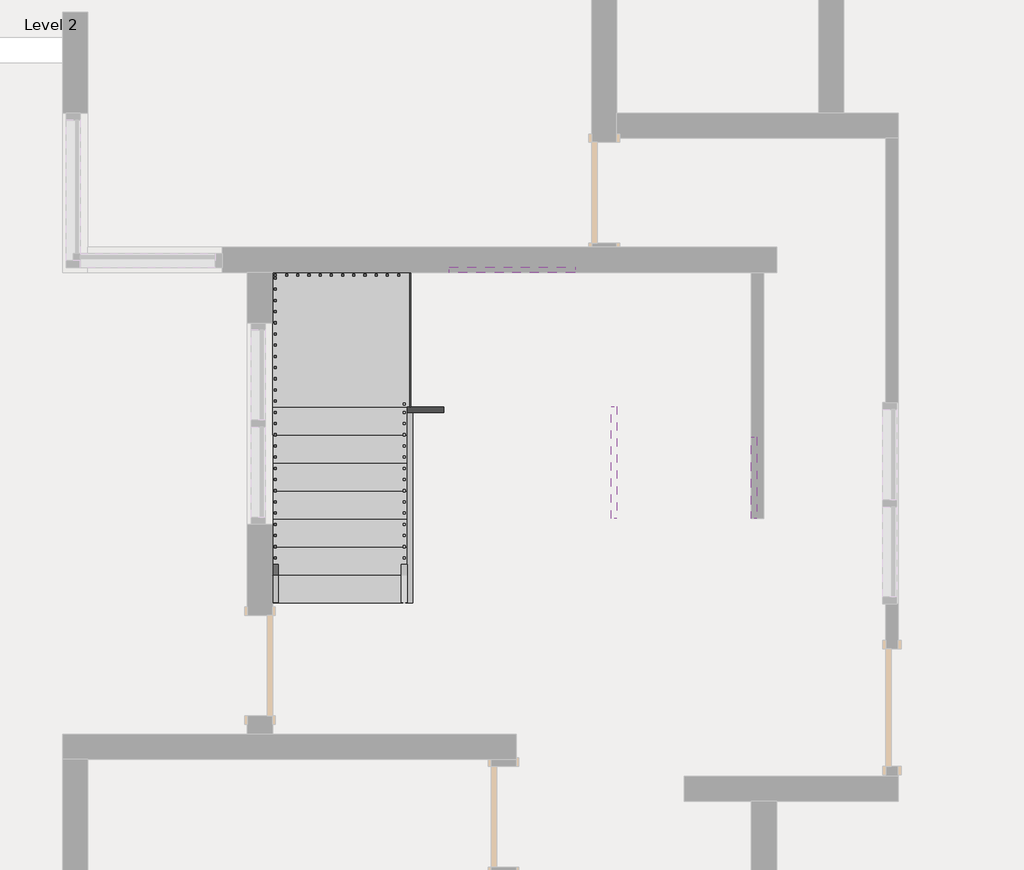
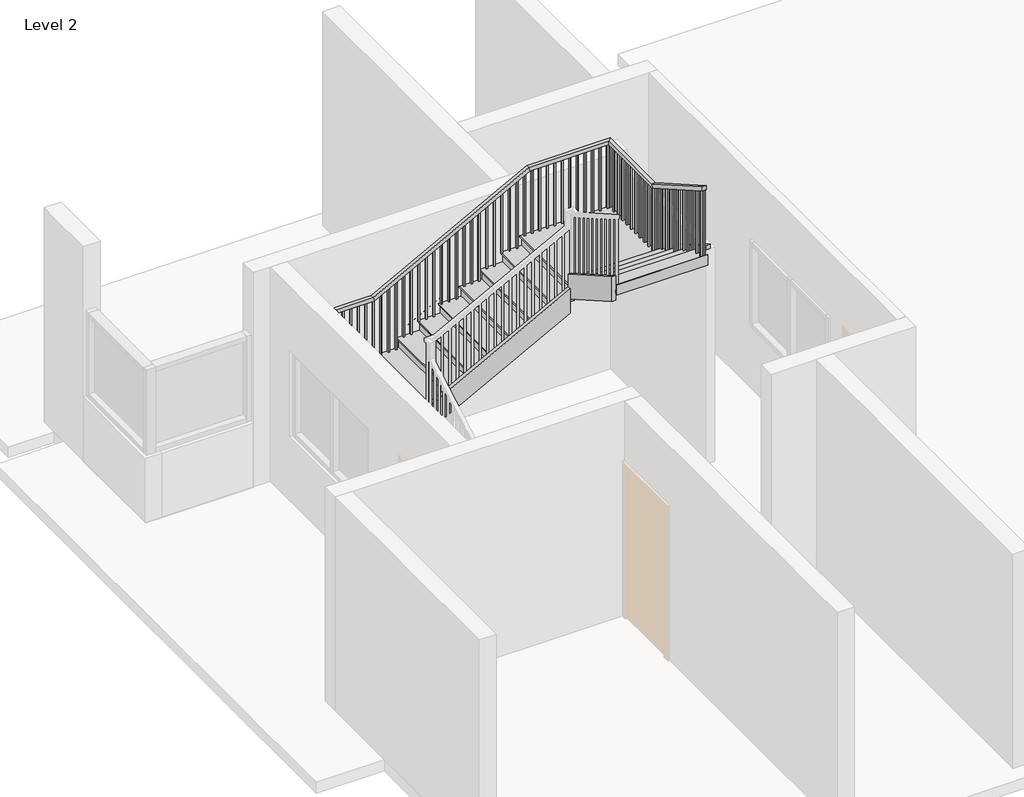
# One storey, part 5 of 5: 6 members, 1 railing, 1 stair flight.
"""IFC4 building model written with IfcOpenShell, lengths in millimetres."""

from ifc_helpers import new_model, si_unit, frame, origin, place, context, project, spatial, polyline, outline, extrude, faceted_brep, transform, mapped, element, save
from components import stair_flight_6f949d0f

model = new_model("IFC4")

# Units and contexts
model_context = context("Model", 3, world=origin())
ifc_project = project(units=[si_unit("LENGTHUNIT", "METRE", prefix="MILLI")], contexts=[model_context])

# Site, building, storey
site = spatial("IfcSite", under=ifc_project)
building = spatial("IfcBuilding", under=site)
storey = spatial("IfcBuildingStorey", under=building, Name="Level 2", Elevation=3048.0)

# Members
placement = place(None, origin())
element("IfcMember", 1, ObjectType="Stringer - 2\" Width", at=placement, inside=storey, context=model_context, shape_type="SweptSolid", body=[
    extrude(outline(polyline([(12459.3864709, 3048.0), (12459.3864709, 3256.974685), (13347.8057723, 3764.6428571), (13962.1498127, 3764.6428571), (12708.0248127, 3048.0), (12459.3864709, 3048.0)])), frame((-41052.5146233, 0.0, 0.0), z_axis=(1.0, 0.0, 0.0), x_axis=(0.0, 1.0, 0.0)), (0.0, 0.0, 1.0), 50.8),
])
element("IfcMember", 2, ObjectType="Stringer - 2\" Width", at=placement, inside=storey, context=model_context, shape_type="SweptSolid", body=[
    extrude(outline(polyline([(4618.6066619, -38752.8324895), (4882.574685, -38257.8924462), (4882.574685, -38905.5924462), (4618.6066619, -39400.5324895), (4618.6066619, -38752.8324895)])), frame((0.0, 15456.5864709, 0.0), z_axis=(0.0, 1.0, 0.0), x_axis=(0.0, 0.0, 1.0)), (0.0, 0.0, 1.0), 50.8),
])
element("IfcMember", 3, ObjectType="Stringer - 2\" Width", at=placement, inside=storey, context=model_context, shape_type="SweptSolid", body=[
    extrude(outline(polyline([(13349.3031292, 5735.6828571), (13221.3864709, 5808.7780904), (13221.3864709, 6159.8318278), (13963.6471696, 5735.6828571), (13349.3031292, 5735.6828571)])), frame((-36658.3146233, 0.0, 0.0), z_axis=(1.0, 0.0, 0.0), x_axis=(0.0, 1.0, 0.0)), (0.0, 0.0, 1.0), 50.8),
])
element("IfcMember", 4, ObjectType="Stringer - 2\" Width", at=placement, inside=storey, context=model_context, shape_type="SweptSolid", body=[
    extrude(outline(polyline([(12459.3864709, 3048.0), (12459.3864709, 3256.974685), (14186.5864709, 4243.9461135), (14186.5864709, 3892.8923761), (12708.0248127, 3048.0), (12459.3864709, 3048.0)])), frame((-39782.5146233, 0.0, 0.0), z_axis=(1.0, 0.0, 0.0), x_axis=(0.0, 1.0, 0.0)), (0.0, 0.0, 1.0), 50.8),
])
element("IfcMember", 5, ObjectType="Stringer - 2\" Width", at=placement, inside=storey, context=model_context, shape_type="SweptSolid", body=[
    extrude(outline(polyline([(4414.8828571, -39782.5146233), (4069.4428571, -39782.5146233), (5058.3495238, -37928.3146233), (5403.7895238, -37928.3146233), (4414.8828571, -39782.5146233)])), frame((0.0, 14186.5864709, 0.0), z_axis=(0.0, 1.0, 0.0), x_axis=(0.0, 0.0, 1.0)), (0.0, 0.0, 1.0), 50.8),
])
element("IfcMember", 6, ObjectType="Stringer - 2\" Width", at=placement, inside=storey, context=model_context, shape_type="SweptSolid", body=[
    extrude(outline(polyline([(14237.3864709, 5579.2603992), (14237.3864709, 5228.2066619), (13221.3864709, 5808.7780904), (13221.3864709, 6159.8318278), (14237.3864709, 5579.2603992)])), frame((-37928.3146233, 0.0, 0.0), z_axis=(1.0, 0.0, 0.0), x_axis=(0.0, 1.0, 0.0)), (0.0, 0.0, 1.0), 50.8),
])

# Railing
element("IfcRailing", 7, ObjectType="Handrail - Rectangular", at=placement, inside=storey, context=model_context, shape_type="SolidModel", body=[
    faceted_brep([(-41001.7146233, 12459.3864709, 4107.5428571), (-41001.7146233, 12459.3864709, 4049.0339009), (-40950.9146233, 12459.3864709, 4049.0339009), (-40950.9146233, 12459.3864709, 4107.5428571), (-41001.7146233, 14404.1798043, 5218.8533333), (-41001.7146233, 14417.6704777, 5168.0533333), (-40950.9146233, 14417.6704777, 5168.0533333), (-40950.9146233, 14404.1798043, 5218.8533333), (-41001.7146233, 15456.5864709, 5218.8533333), (-41001.7146233, 15456.5864709, 5168.0533333), (-40950.9146233, 15405.7864709, 5168.0533333), (-40950.9146233, 15405.7864709, 5218.8533333), (-39875.9503376, 15456.5864709, 5218.8533333), (-39863.2503376, 15456.5864709, 5168.0533333), (-39863.2503376, 15405.7864709, 5168.0533333), (-39875.9503376, 15405.7864709, 5218.8533333), (-37784.0789091, 15456.5864709, 6334.5180952), (-37771.3789091, 15456.5864709, 6283.7180952), (-37771.3789091, 15405.7864709, 6283.7180952), (-37784.0789091, 15405.7864709, 6334.5180952), (-36658.3146233, 15456.5864709, 6334.5180952), (-36658.3146233, 15456.5864709, 6283.7180952), (-36709.1146233, 15405.7864709, 6283.7180952), (-36709.1146233, 15405.7864709, 6334.5180952), (-36658.3146233, 14404.1798043, 6334.5180952), (-36658.3146233, 14390.6891309, 6283.7180952), (-36709.1146233, 14390.6891309, 6283.7180952), (-36709.1146233, 14404.1798043, 6334.5180952), (-36658.3146233, 13221.3864709, 7010.4), (-36709.1146233, 13221.3864709, 7010.4), (-36709.1146233, 13221.3864709, 6951.8910438), (-36658.3146233, 13221.3864709, 6951.8910438)], [[[0, 1, 2, 3]], [[1, 0, 4, 5]], [[2, 1, 5, 6]], [[3, 2, 6, 7]], [[0, 3, 7, 4]], [[5, 4, 8, 9]], [[6, 5, 9, 10]], [[7, 6, 10, 11]], [[4, 7, 11, 8]], [[9, 8, 12, 13]], [[10, 9, 13, 14]], [[11, 10, 14, 15]], [[8, 11, 15, 12]], [[13, 12, 16, 17]], [[14, 13, 17, 18]], [[15, 14, 18, 19]], [[12, 15, 19, 16]], [[17, 16, 20, 21]], [[18, 17, 21, 22]], [[19, 18, 22, 23]], [[16, 19, 23, 20]], [[21, 20, 24, 25]], [[22, 21, 25, 26]], [[23, 22, 26, 27]], [[20, 23, 27, 24]], [[28, 29, 30, 31]], [[25, 24, 28, 31]], [[26, 25, 31, 30]], [[27, 26, 30, 29]], [[24, 27, 29, 28]]]),
    extrude(outline(polyline([(13307.1114709, 6902.9053295), (13307.1114709, 5950.8571429), (13288.0614709, 5950.8571429), (13288.0614709, 6913.7910438), (13307.1114709, 6902.9053295)])), frame((-36693.2396233, 0.0, 0.0), z_axis=(1.0, 0.0, 0.0), x_axis=(0.0, 1.0, 0.0)), (0.0, 0.0, 1.0), 19.05),
    extrude(outline(polyline([(13408.7114709, 6844.8481866), (13408.7114709, 5950.8571429), (13389.6614709, 5950.8571429), (13389.6614709, 6855.7339009), (13408.7114709, 6844.8481866)])), frame((-36693.2396233, 0.0, 0.0), z_axis=(1.0, 0.0, 0.0), x_axis=(0.0, 1.0, 0.0)), (0.0, 0.0, 1.0), 19.05),
    extrude(outline(polyline([(13510.3114709, 6786.7910438), (13510.3114709, 5805.7142857), (13491.2614709, 5805.7142857), (13491.2614709, 6797.6767581), (13510.3114709, 6786.7910438)])), frame((-36693.2396233, 0.0, 0.0), z_axis=(1.0, 0.0, 0.0), x_axis=(0.0, 1.0, 0.0)), (0.0, 0.0, 1.0), 19.05),
    extrude(outline(polyline([(13611.9114709, 6728.7339009), (13611.9114709, 5805.7142857), (13592.8614709, 5805.7142857), (13592.8614709, 6739.6196152), (13611.9114709, 6728.7339009)])), frame((-36693.2396233, 0.0, 0.0), z_axis=(1.0, 0.0, 0.0), x_axis=(0.0, 1.0, 0.0)), (0.0, 0.0, 1.0), 19.05),
    extrude(outline(polyline([(13713.5114709, 6670.6767581), (13713.5114709, 5805.7142857), (13694.4614709, 5805.7142857), (13694.4614709, 6681.5624723), (13713.5114709, 6670.6767581)])), frame((-36693.2396233, 0.0, 0.0), z_axis=(1.0, 0.0, 0.0), x_axis=(0.0, 1.0, 0.0)), (0.0, 0.0, 1.0), 19.05),
    extrude(outline(polyline([(13815.1114709, 6612.6196152), (13815.1114709, 5660.5714286), (13796.0614709, 5660.5714286), (13796.0614709, 6623.5053295), (13815.1114709, 6612.6196152)])), frame((-36693.2396233, 0.0, 0.0), z_axis=(1.0, 0.0, 0.0), x_axis=(0.0, 1.0, 0.0)), (0.0, 0.0, 1.0), 19.05),
    extrude(outline(polyline([(13916.7114709, 6554.5624723), (13916.7114709, 5660.5714286), (13897.6614709, 5660.5714286), (13897.6614709, 6565.4481866), (13916.7114709, 6554.5624723)])), frame((-36693.2396233, 0.0, 0.0), z_axis=(1.0, 0.0, 0.0), x_axis=(0.0, 1.0, 0.0)), (0.0, 0.0, 1.0), 19.05),
    extrude(outline(polyline([(14018.3114709, 6496.5053295), (14018.3114709, 5515.4285714), (13999.2614709, 5515.4285714), (13999.2614709, 6507.3910438), (14018.3114709, 6496.5053295)])), frame((-36693.2396233, 0.0, 0.0), z_axis=(1.0, 0.0, 0.0), x_axis=(0.0, 1.0, 0.0)), (0.0, 0.0, 1.0), 19.05),
    extrude(outline(polyline([(14119.9114709, 6438.4481866), (14119.9114709, 5515.4285714), (14100.8614709, 5515.4285714), (14100.8614709, 6449.3339009), (14119.9114709, 6438.4481866)])), frame((-36693.2396233, 0.0, 0.0), z_axis=(1.0, 0.0, 0.0), x_axis=(0.0, 1.0, 0.0)), (0.0, 0.0, 1.0), 19.05),
    extrude(outline(polyline([(14221.5114709, 6380.3910438), (14221.5114709, 5515.4285714), (14202.4614709, 5515.4285714), (14202.4614709, 6391.2767581), (14221.5114709, 6380.3910438)])), frame((-36693.2396233, 0.0, 0.0), z_axis=(1.0, 0.0, 0.0), x_axis=(0.0, 1.0, 0.0)), (0.0, 0.0, 1.0), 19.05),
    extrude(outline(polyline([(14323.1114709, 6322.3339009), (14323.1114709, 5370.2857143), (14304.0614709, 5370.2857143), (14304.0614709, 6333.2196152), (14323.1114709, 6322.3339009)])), frame((-36693.2396233, 0.0, 0.0), z_axis=(1.0, 0.0, 0.0), x_axis=(0.0, 1.0, 0.0)), (0.0, 0.0, 1.0), 19.05),
    extrude(outline(polyline([(-36674.1896233, 14424.7114709), (-36674.1896233, 14405.6614709), (-36693.2396233, 14405.6614709), (-36693.2396233, 14424.7114709), (-36674.1896233, 14424.7114709)])), frame((0.0, 0.0, 5370.2857143), z_axis=(0.0, 0.0, 1.0), x_axis=(1.0, 0.0, 0.0)), (0.0, 0.0, 1.0), 913.432381),
    extrude(outline(polyline([(-36674.1896233, 14526.3114709), (-36674.1896233, 14507.2614709), (-36693.2396233, 14507.2614709), (-36693.2396233, 14526.3114709), (-36674.1896233, 14526.3114709)])), frame((0.0, 0.0, 5370.2857143), z_axis=(0.0, 0.0, 1.0), x_axis=(1.0, 0.0, 0.0)), (0.0, 0.0, 1.0), 913.432381),
    extrude(outline(polyline([(-36674.1896233, 14627.9114709), (-36674.1896233, 14608.8614709), (-36693.2396233, 14608.8614709), (-36693.2396233, 14627.9114709), (-36674.1896233, 14627.9114709)])), frame((0.0, 0.0, 5370.2857143), z_axis=(0.0, 0.0, 1.0), x_axis=(1.0, 0.0, 0.0)), (0.0, 0.0, 1.0), 913.432381),
    extrude(outline(polyline([(-36674.1896233, 14729.5114709), (-36674.1896233, 14710.4614709), (-36693.2396233, 14710.4614709), (-36693.2396233, 14729.5114709), (-36674.1896233, 14729.5114709)])), frame((0.0, 0.0, 5370.2857143), z_axis=(0.0, 0.0, 1.0), x_axis=(1.0, 0.0, 0.0)), (0.0, 0.0, 1.0), 913.432381),
    extrude(outline(polyline([(-36674.1896233, 14831.1114709), (-36674.1896233, 14812.0614709), (-36693.2396233, 14812.0614709), (-36693.2396233, 14831.1114709), (-36674.1896233, 14831.1114709)])), frame((0.0, 0.0, 5370.2857143), z_axis=(0.0, 0.0, 1.0), x_axis=(1.0, 0.0, 0.0)), (0.0, 0.0, 1.0), 913.432381),
    extrude(outline(polyline([(-36674.1896233, 14932.7114709), (-36674.1896233, 14913.6614709), (-36693.2396233, 14913.6614709), (-36693.2396233, 14932.7114709), (-36674.1896233, 14932.7114709)])), frame((0.0, 0.0, 5370.2857143), z_axis=(0.0, 0.0, 1.0), x_axis=(1.0, 0.0, 0.0)), (0.0, 0.0, 1.0), 913.432381),
    extrude(outline(polyline([(-36674.1896233, 15034.3114709), (-36674.1896233, 15015.2614709), (-36693.2396233, 15015.2614709), (-36693.2396233, 15034.3114709), (-36674.1896233, 15034.3114709)])), frame((0.0, 0.0, 5370.2857143), z_axis=(0.0, 0.0, 1.0), x_axis=(1.0, 0.0, 0.0)), (0.0, 0.0, 1.0), 913.432381),
    extrude(outline(polyline([(-36674.1896233, 15135.9114709), (-36674.1896233, 15116.8614709), (-36693.2396233, 15116.8614709), (-36693.2396233, 15135.9114709), (-36674.1896233, 15135.9114709)])), frame((0.0, 0.0, 5370.2857143), z_axis=(0.0, 0.0, 1.0), x_axis=(1.0, 0.0, 0.0)), (0.0, 0.0, 1.0), 913.432381),
    extrude(outline(polyline([(-36674.1896233, 15237.5114709), (-36674.1896233, 15218.4614709), (-36693.2396233, 15218.4614709), (-36693.2396233, 15237.5114709), (-36674.1896233, 15237.5114709)])), frame((0.0, 0.0, 5370.2857143), z_axis=(0.0, 0.0, 1.0), x_axis=(1.0, 0.0, 0.0)), (0.0, 0.0, 1.0), 913.432381),
    extrude(outline(polyline([(-36674.1896233, 15339.1114709), (-36674.1896233, 15320.0614709), (-36693.2396233, 15320.0614709), (-36693.2396233, 15339.1114709), (-36674.1896233, 15339.1114709)])), frame((0.0, 0.0, 5370.2857143), z_axis=(0.0, 0.0, 1.0), x_axis=(1.0, 0.0, 0.0)), (0.0, 0.0, 1.0), 913.432381),
    extrude(outline(polyline([(-36718.6396233, 15440.7114709), (-36699.5896233, 15440.7114709), (-36699.5896233, 15421.6614709), (-36718.6396233, 15421.6614709), (-36718.6396233, 15440.7114709)])), frame((0.0, 0.0, 5370.2857143), z_axis=(0.0, 0.0, 1.0), x_axis=(1.0, 0.0, 0.0)), (0.0, 0.0, 1.0), 913.432381),
    extrude(outline(polyline([(-36820.2396233, 15440.7114709), (-36801.1896233, 15440.7114709), (-36801.1896233, 15421.6614709), (-36820.2396233, 15421.6614709), (-36820.2396233, 15440.7114709)])), frame((0.0, 0.0, 5370.2857143), z_axis=(0.0, 0.0, 1.0), x_axis=(1.0, 0.0, 0.0)), (0.0, 0.0, 1.0), 913.432381),
    extrude(outline(polyline([(-36921.8396233, 15440.7114709), (-36902.7896233, 15440.7114709), (-36902.7896233, 15421.6614709), (-36921.8396233, 15421.6614709), (-36921.8396233, 15440.7114709)])), frame((0.0, 0.0, 5370.2857143), z_axis=(0.0, 0.0, 1.0), x_axis=(1.0, 0.0, 0.0)), (0.0, 0.0, 1.0), 913.432381),
    extrude(outline(polyline([(-37023.4396233, 15440.7114709), (-37004.3896233, 15440.7114709), (-37004.3896233, 15421.6614709), (-37023.4396233, 15421.6614709), (-37023.4396233, 15440.7114709)])), frame((0.0, 0.0, 5370.2857143), z_axis=(0.0, 0.0, 1.0), x_axis=(1.0, 0.0, 0.0)), (0.0, 0.0, 1.0), 913.432381),
    extrude(outline(polyline([(-37125.0396233, 15440.7114709), (-37105.9896233, 15440.7114709), (-37105.9896233, 15421.6614709), (-37125.0396233, 15421.6614709), (-37125.0396233, 15440.7114709)])), frame((0.0, 0.0, 5370.2857143), z_axis=(0.0, 0.0, 1.0), x_axis=(1.0, 0.0, 0.0)), (0.0, 0.0, 1.0), 913.432381),
    extrude(outline(polyline([(-37226.6396233, 15440.7114709), (-37207.5896233, 15440.7114709), (-37207.5896233, 15421.6614709), (-37226.6396233, 15421.6614709), (-37226.6396233, 15440.7114709)])), frame((0.0, 0.0, 5370.2857143), z_axis=(0.0, 0.0, 1.0), x_axis=(1.0, 0.0, 0.0)), (0.0, 0.0, 1.0), 913.432381),
    extrude(outline(polyline([(-37328.2396233, 15440.7114709), (-37309.1896233, 15440.7114709), (-37309.1896233, 15421.6614709), (-37328.2396233, 15421.6614709), (-37328.2396233, 15440.7114709)])), frame((0.0, 0.0, 5370.2857143), z_axis=(0.0, 0.0, 1.0), x_axis=(1.0, 0.0, 0.0)), (0.0, 0.0, 1.0), 913.432381),
    extrude(outline(polyline([(-37429.8396233, 15440.7114709), (-37410.7896233, 15440.7114709), (-37410.7896233, 15421.6614709), (-37429.8396233, 15421.6614709), (-37429.8396233, 15440.7114709)])), frame((0.0, 0.0, 5370.2857143), z_axis=(0.0, 0.0, 1.0), x_axis=(1.0, 0.0, 0.0)), (0.0, 0.0, 1.0), 913.432381),
    extrude(outline(polyline([(-37531.4396233, 15440.7114709), (-37512.3896233, 15440.7114709), (-37512.3896233, 15421.6614709), (-37531.4396233, 15421.6614709), (-37531.4396233, 15440.7114709)])), frame((0.0, 0.0, 5370.2857143), z_axis=(0.0, 0.0, 1.0), x_axis=(1.0, 0.0, 0.0)), (0.0, 0.0, 1.0), 913.432381),
    extrude(outline(polyline([(-37633.0396233, 15440.7114709), (-37613.9896233, 15440.7114709), (-37613.9896233, 15421.6614709), (-37633.0396233, 15421.6614709), (-37633.0396233, 15440.7114709)])), frame((0.0, 0.0, 5370.2857143), z_axis=(0.0, 0.0, 1.0), x_axis=(1.0, 0.0, 0.0)), (0.0, 0.0, 1.0), 913.432381),
    extrude(outline(polyline([(-37734.6396233, 15440.7114709), (-37715.5896233, 15440.7114709), (-37715.5896233, 15421.6614709), (-37734.6396233, 15421.6614709), (-37734.6396233, 15440.7114709)])), frame((0.0, 0.0, 5370.2857143), z_axis=(0.0, 0.0, 1.0), x_axis=(1.0, 0.0, 0.0)), (0.0, 0.0, 1.0), 913.432381),
    extrude(outline(polyline([(6249.1257143, -37836.2396233), (5370.2857143, -37836.2396233), (5370.2857143, -37817.1896233), (6259.2857143, -37817.1896233), (6249.1257143, -37836.2396233)])), frame((0.0, 15421.6614709, 0.0), z_axis=(0.0, 1.0, 0.0), x_axis=(0.0, 0.0, 1.0)), (0.0, 0.0, 1.0), 19.05),
    extrude(outline(polyline([(6194.9390476, -37937.8396233), (5225.1428571, -37937.8396233), (5225.1428571, -37918.7896233), (6205.0990476, -37918.7896233), (6194.9390476, -37937.8396233)])), frame((0.0, 15421.6614709, 0.0), z_axis=(0.0, 1.0, 0.0), x_axis=(0.0, 0.0, 1.0)), (0.0, 0.0, 1.0), 19.05),
    extrude(outline(polyline([(6140.752381, -38039.4396233), (5225.1428571, -38039.4396233), (5225.1428571, -38020.3896233), (6150.912381, -38020.3896233), (6140.752381, -38039.4396233)])), frame((0.0, 15421.6614709, 0.0), z_axis=(0.0, 1.0, 0.0), x_axis=(0.0, 0.0, 1.0)), (0.0, 0.0, 1.0), 19.05),
    extrude(outline(polyline([(6086.5657143, -38141.0396233), (5225.1428571, -38141.0396233), (5225.1428571, -38121.9896233), (6096.7257143, -38121.9896233), (6086.5657143, -38141.0396233)])), frame((0.0, 15421.6614709, 0.0), z_axis=(0.0, 1.0, 0.0), x_axis=(0.0, 0.0, 1.0)), (0.0, 0.0, 1.0), 19.05),
    extrude(outline(polyline([(6032.3790476, -38242.6396233), (5080.0, -38242.6396233), (5080.0, -38223.5896233), (6042.5390476, -38223.5896233), (6032.3790476, -38242.6396233)])), frame((0.0, 15421.6614709, 0.0), z_axis=(0.0, 1.0, 0.0), x_axis=(0.0, 0.0, 1.0)), (0.0, 0.0, 1.0), 19.05),
    extrude(outline(polyline([(5978.192381, -38344.2396233), (5080.0, -38344.2396233), (5080.0, -38325.1896233), (5988.352381, -38325.1896233), (5978.192381, -38344.2396233)])), frame((0.0, 15421.6614709, 0.0), z_axis=(0.0, 1.0, 0.0), x_axis=(0.0, 0.0, 1.0)), (0.0, 0.0, 1.0), 19.05),
    extrude(outline(polyline([(5924.0057143, -38445.8396233), (4934.8571429, -38445.8396233), (4934.8571429, -38426.7896233), (5934.1657143, -38426.7896233), (5924.0057143, -38445.8396233)])), frame((0.0, 15421.6614709, 0.0), z_axis=(0.0, 1.0, 0.0), x_axis=(0.0, 0.0, 1.0)), (0.0, 0.0, 1.0), 19.05),
    extrude(outline(polyline([(5869.8190476, -38547.4396233), (4934.8571429, -38547.4396233), (4934.8571429, -38528.3896233), (5879.9790476, -38528.3896233), (5869.8190476, -38547.4396233)])), frame((0.0, 15421.6614709, 0.0), z_axis=(0.0, 1.0, 0.0), x_axis=(0.0, 0.0, 1.0)), (0.0, 0.0, 1.0), 19.05),
    extrude(outline(polyline([(5815.632381, -38649.0396233), (4934.8571429, -38649.0396233), (4934.8571429, -38629.9896233), (5825.792381, -38629.9896233), (5815.632381, -38649.0396233)])), frame((0.0, 15421.6614709, 0.0), z_axis=(0.0, 1.0, 0.0), x_axis=(0.0, 0.0, 1.0)), (0.0, 0.0, 1.0), 19.05),
    extrude(outline(polyline([(5761.4457143, -38750.6396233), (4789.7142857, -38750.6396233), (4789.7142857, -38731.5896233), (5771.6057143, -38731.5896233), (5761.4457143, -38750.6396233)])), frame((0.0, 15421.6614709, 0.0), z_axis=(0.0, 1.0, 0.0), x_axis=(0.0, 0.0, 1.0)), (0.0, 0.0, 1.0), 19.05),
    extrude(outline(polyline([(5707.2590476, -38852.2396233), (4789.7142857, -38852.2396233), (4789.7142857, -38833.1896233), (5717.4190476, -38833.1896233), (5707.2590476, -38852.2396233)])), frame((0.0, 15421.6614709, 0.0), z_axis=(0.0, 1.0, 0.0), x_axis=(0.0, 0.0, 1.0)), (0.0, 0.0, 1.0), 19.05),
    extrude(outline(polyline([(5653.072381, -38953.8396233), (4789.7142857, -38953.8396233), (4789.7142857, -38934.7896233), (5663.232381, -38934.7896233), (5653.072381, -38953.8396233)])), frame((0.0, 15421.6614709, 0.0), z_axis=(0.0, 1.0, 0.0), x_axis=(0.0, 0.0, 1.0)), (0.0, 0.0, 1.0), 19.05),
    extrude(outline(polyline([(5598.8857143, -39055.4396233), (4644.5714286, -39055.4396233), (4644.5714286, -39036.3896233), (5609.0457143, -39036.3896233), (5598.8857143, -39055.4396233)])), frame((0.0, 15421.6614709, 0.0), z_axis=(0.0, 1.0, 0.0), x_axis=(0.0, 0.0, 1.0)), (0.0, 0.0, 1.0), 19.05),
    extrude(outline(polyline([(5544.6990476, -39157.0396233), (4644.5714286, -39157.0396233), (4644.5714286, -39137.9896233), (5554.8590476, -39137.9896233), (5544.6990476, -39157.0396233)])), frame((0.0, 15421.6614709, 0.0), z_axis=(0.0, 1.0, 0.0), x_axis=(0.0, 0.0, 1.0)), (0.0, 0.0, 1.0), 19.05),
    extrude(outline(polyline([(5490.512381, -39258.6396233), (4644.5714286, -39258.6396233), (4644.5714286, -39239.5896233), (5500.672381, -39239.5896233), (5490.512381, -39258.6396233)])), frame((0.0, 15421.6614709, 0.0), z_axis=(0.0, 1.0, 0.0), x_axis=(0.0, 0.0, 1.0)), (0.0, 0.0, 1.0), 19.05),
    extrude(outline(polyline([(5436.3257143, -39360.2396233), (4499.4285714, -39360.2396233), (4499.4285714, -39341.1896233), (5446.4857143, -39341.1896233), (5436.3257143, -39360.2396233)])), frame((0.0, 15421.6614709, 0.0), z_axis=(0.0, 1.0, 0.0), x_axis=(0.0, 0.0, 1.0)), (0.0, 0.0, 1.0), 19.05),
    extrude(outline(polyline([(5382.1390476, -39461.8396233), (4499.4285714, -39461.8396233), (4499.4285714, -39442.7896233), (5392.2990476, -39442.7896233), (5382.1390476, -39461.8396233)])), frame((0.0, 15421.6614709, 0.0), z_axis=(0.0, 1.0, 0.0), x_axis=(0.0, 0.0, 1.0)), (0.0, 0.0, 1.0), 19.05),
    extrude(outline(polyline([(5327.952381, -39563.4396233), (4354.2857143, -39563.4396233), (4354.2857143, -39544.3896233), (5338.112381, -39544.3896233), (5327.952381, -39563.4396233)])), frame((0.0, 15421.6614709, 0.0), z_axis=(0.0, 1.0, 0.0), x_axis=(0.0, 0.0, 1.0)), (0.0, 0.0, 1.0), 19.05),
    extrude(outline(polyline([(5273.7657143, -39665.0396233), (4354.2857143, -39665.0396233), (4354.2857143, -39645.9896233), (5283.9257143, -39645.9896233), (5273.7657143, -39665.0396233)])), frame((0.0, 15421.6614709, 0.0), z_axis=(0.0, 1.0, 0.0), x_axis=(0.0, 0.0, 1.0)), (0.0, 0.0, 1.0), 19.05),
    extrude(outline(polyline([(5219.5790476, -39766.6396233), (4354.2857143, -39766.6396233), (4354.2857143, -39747.5896233), (5229.7390476, -39747.5896233), (5219.5790476, -39766.6396233)])), frame((0.0, 15421.6614709, 0.0), z_axis=(0.0, 1.0, 0.0), x_axis=(0.0, 0.0, 1.0)), (0.0, 0.0, 1.0), 19.05),
    extrude(outline(polyline([(5165.392381, -39868.2396233), (4209.1428571, -39868.2396233), (4209.1428571, -39849.1896233), (5175.552381, -39849.1896233), (5165.392381, -39868.2396233)])), frame((0.0, 15421.6614709, 0.0), z_axis=(0.0, 1.0, 0.0), x_axis=(0.0, 0.0, 1.0)), (0.0, 0.0, 1.0), 19.05),
    extrude(outline(polyline([(-39969.8396233, 15440.7114709), (-39950.7896233, 15440.7114709), (-39950.7896233, 15421.6614709), (-39969.8396233, 15421.6614709), (-39969.8396233, 15440.7114709)])), frame((0.0, 0.0, 4209.1428571), z_axis=(0.0, 0.0, 1.0), x_axis=(1.0, 0.0, 0.0)), (0.0, 0.0, 1.0), 958.9104762),
    extrude(outline(polyline([(-40071.4396233, 15440.7114709), (-40052.3896233, 15440.7114709), (-40052.3896233, 15421.6614709), (-40071.4396233, 15421.6614709), (-40071.4396233, 15440.7114709)])), frame((0.0, 0.0, 4209.1428571), z_axis=(0.0, 0.0, 1.0), x_axis=(1.0, 0.0, 0.0)), (0.0, 0.0, 1.0), 958.9104762),
    extrude(outline(polyline([(-40173.0396233, 15440.7114709), (-40153.9896233, 15440.7114709), (-40153.9896233, 15421.6614709), (-40173.0396233, 15421.6614709), (-40173.0396233, 15440.7114709)])), frame((0.0, 0.0, 4209.1428571), z_axis=(0.0, 0.0, 1.0), x_axis=(1.0, 0.0, 0.0)), (0.0, 0.0, 1.0), 958.9104762),
    extrude(outline(polyline([(-40274.6396233, 15440.7114709), (-40255.5896233, 15440.7114709), (-40255.5896233, 15421.6614709), (-40274.6396233, 15421.6614709), (-40274.6396233, 15440.7114709)])), frame((0.0, 0.0, 4209.1428571), z_axis=(0.0, 0.0, 1.0), x_axis=(1.0, 0.0, 0.0)), (0.0, 0.0, 1.0), 958.9104762),
    extrude(outline(polyline([(-40376.2396233, 15440.7114709), (-40357.1896233, 15440.7114709), (-40357.1896233, 15421.6614709), (-40376.2396233, 15421.6614709), (-40376.2396233, 15440.7114709)])), frame((0.0, 0.0, 4209.1428571), z_axis=(0.0, 0.0, 1.0), x_axis=(1.0, 0.0, 0.0)), (0.0, 0.0, 1.0), 958.9104762),
    extrude(outline(polyline([(-40477.8396233, 15440.7114709), (-40458.7896233, 15440.7114709), (-40458.7896233, 15421.6614709), (-40477.8396233, 15421.6614709), (-40477.8396233, 15440.7114709)])), frame((0.0, 0.0, 4209.1428571), z_axis=(0.0, 0.0, 1.0), x_axis=(1.0, 0.0, 0.0)), (0.0, 0.0, 1.0), 958.9104762),
    extrude(outline(polyline([(-40579.4396233, 15440.7114709), (-40560.3896233, 15440.7114709), (-40560.3896233, 15421.6614709), (-40579.4396233, 15421.6614709), (-40579.4396233, 15440.7114709)])), frame((0.0, 0.0, 4209.1428571), z_axis=(0.0, 0.0, 1.0), x_axis=(1.0, 0.0, 0.0)), (0.0, 0.0, 1.0), 958.9104762),
    extrude(outline(polyline([(-40681.0396233, 15440.7114709), (-40661.9896233, 15440.7114709), (-40661.9896233, 15421.6614709), (-40681.0396233, 15421.6614709), (-40681.0396233, 15440.7114709)])), frame((0.0, 0.0, 4209.1428571), z_axis=(0.0, 0.0, 1.0), x_axis=(1.0, 0.0, 0.0)), (0.0, 0.0, 1.0), 958.9104762),
    extrude(outline(polyline([(-40782.6396233, 15440.7114709), (-40763.5896233, 15440.7114709), (-40763.5896233, 15421.6614709), (-40782.6396233, 15421.6614709), (-40782.6396233, 15440.7114709)])), frame((0.0, 0.0, 4209.1428571), z_axis=(0.0, 0.0, 1.0), x_axis=(1.0, 0.0, 0.0)), (0.0, 0.0, 1.0), 958.9104762),
    extrude(outline(polyline([(-40884.2396233, 15440.7114709), (-40865.1896233, 15440.7114709), (-40865.1896233, 15421.6614709), (-40884.2396233, 15421.6614709), (-40884.2396233, 15440.7114709)])), frame((0.0, 0.0, 4209.1428571), z_axis=(0.0, 0.0, 1.0), x_axis=(1.0, 0.0, 0.0)), (0.0, 0.0, 1.0), 958.9104762),
    extrude(outline(polyline([(-40985.8396233, 15396.2614709), (-40985.8396233, 15415.3114709), (-40966.7896233, 15415.3114709), (-40966.7896233, 15396.2614709), (-40985.8396233, 15396.2614709)])), frame((0.0, 0.0, 4209.1428571), z_axis=(0.0, 0.0, 1.0), x_axis=(1.0, 0.0, 0.0)), (0.0, 0.0, 1.0), 958.9104762),
    extrude(outline(polyline([(-40985.8396233, 15294.6614709), (-40985.8396233, 15313.7114709), (-40966.7896233, 15313.7114709), (-40966.7896233, 15294.6614709), (-40985.8396233, 15294.6614709)])), frame((0.0, 0.0, 4209.1428571), z_axis=(0.0, 0.0, 1.0), x_axis=(1.0, 0.0, 0.0)), (0.0, 0.0, 1.0), 958.9104762),
    extrude(outline(polyline([(-40985.8396233, 15193.0614709), (-40985.8396233, 15212.1114709), (-40966.7896233, 15212.1114709), (-40966.7896233, 15193.0614709), (-40985.8396233, 15193.0614709)])), frame((0.0, 0.0, 4209.1428571), z_axis=(0.0, 0.0, 1.0), x_axis=(1.0, 0.0, 0.0)), (0.0, 0.0, 1.0), 958.9104762),
    extrude(outline(polyline([(-40985.8396233, 15091.4614709), (-40985.8396233, 15110.5114709), (-40966.7896233, 15110.5114709), (-40966.7896233, 15091.4614709), (-40985.8396233, 15091.4614709)])), frame((0.0, 0.0, 4209.1428571), z_axis=(0.0, 0.0, 1.0), x_axis=(1.0, 0.0, 0.0)), (0.0, 0.0, 1.0), 958.9104762),
    extrude(outline(polyline([(-40985.8396233, 14989.8614709), (-40985.8396233, 15008.9114709), (-40966.7896233, 15008.9114709), (-40966.7896233, 14989.8614709), (-40985.8396233, 14989.8614709)])), frame((0.0, 0.0, 4209.1428571), z_axis=(0.0, 0.0, 1.0), x_axis=(1.0, 0.0, 0.0)), (0.0, 0.0, 1.0), 958.9104762),
    extrude(outline(polyline([(-40985.8396233, 14888.2614709), (-40985.8396233, 14907.3114709), (-40966.7896233, 14907.3114709), (-40966.7896233, 14888.2614709), (-40985.8396233, 14888.2614709)])), frame((0.0, 0.0, 4209.1428571), z_axis=(0.0, 0.0, 1.0), x_axis=(1.0, 0.0, 0.0)), (0.0, 0.0, 1.0), 958.9104762),
    extrude(outline(polyline([(-40985.8396233, 14786.6614709), (-40985.8396233, 14805.7114709), (-40966.7896233, 14805.7114709), (-40966.7896233, 14786.6614709), (-40985.8396233, 14786.6614709)])), frame((0.0, 0.0, 4209.1428571), z_axis=(0.0, 0.0, 1.0), x_axis=(1.0, 0.0, 0.0)), (0.0, 0.0, 1.0), 958.9104762),
    extrude(outline(polyline([(-40985.8396233, 14685.0614709), (-40985.8396233, 14704.1114709), (-40966.7896233, 14704.1114709), (-40966.7896233, 14685.0614709), (-40985.8396233, 14685.0614709)])), frame((0.0, 0.0, 4209.1428571), z_axis=(0.0, 0.0, 1.0), x_axis=(1.0, 0.0, 0.0)), (0.0, 0.0, 1.0), 958.9104762),
    extrude(outline(polyline([(-40985.8396233, 14583.4614709), (-40985.8396233, 14602.5114709), (-40966.7896233, 14602.5114709), (-40966.7896233, 14583.4614709), (-40985.8396233, 14583.4614709)])), frame((0.0, 0.0, 4209.1428571), z_axis=(0.0, 0.0, 1.0), x_axis=(1.0, 0.0, 0.0)), (0.0, 0.0, 1.0), 958.9104762),
    extrude(outline(polyline([(-40985.8396233, 14481.8614709), (-40985.8396233, 14500.9114709), (-40966.7896233, 14500.9114709), (-40966.7896233, 14481.8614709), (-40985.8396233, 14481.8614709)])), frame((0.0, 0.0, 4209.1428571), z_axis=(0.0, 0.0, 1.0), x_axis=(1.0, 0.0, 0.0)), (0.0, 0.0, 1.0), 958.9104762),
    extrude(outline(polyline([(14399.3114709, 5157.5624723), (14399.3114709, 4209.1428571), (14380.2614709, 4209.1428571), (14380.2614709, 5146.6767581), (14399.3114709, 5157.5624723)])), frame((-40985.8396233, 0.0, 0.0), z_axis=(1.0, 0.0, 0.0), x_axis=(0.0, 1.0, 0.0)), (0.0, 0.0, 1.0), 19.05),
    extrude(outline(polyline([(14297.7114709, 5099.5053295), (14297.7114709, 4209.1428571), (14278.6614709, 4209.1428571), (14278.6614709, 5088.6196152), (14297.7114709, 5099.5053295)])), frame((-40985.8396233, 0.0, 0.0), z_axis=(1.0, 0.0, 0.0), x_axis=(0.0, 1.0, 0.0)), (0.0, 0.0, 1.0), 19.05),
    extrude(outline(polyline([(14196.1114709, 5041.4481866), (14196.1114709, 4064.0), (14177.0614709, 4064.0), (14177.0614709, 5030.5624723), (14196.1114709, 5041.4481866)])), frame((-40985.8396233, 0.0, 0.0), z_axis=(1.0, 0.0, 0.0), x_axis=(0.0, 1.0, 0.0)), (0.0, 0.0, 1.0), 19.05),
    extrude(outline(polyline([(14094.5114709, 4983.3910438), (14094.5114709, 4064.0), (14075.4614709, 4064.0), (14075.4614709, 4972.5053295), (14094.5114709, 4983.3910438)])), frame((-40985.8396233, 0.0, 0.0), z_axis=(1.0, 0.0, 0.0), x_axis=(0.0, 1.0, 0.0)), (0.0, 0.0, 1.0), 19.05),
    extrude(outline(polyline([(13992.9114709, 4925.3339009), (13992.9114709, 4064.0), (13973.8614709, 4064.0), (13973.8614709, 4914.4481866), (13992.9114709, 4925.3339009)])), frame((-40985.8396233, 0.0, 0.0), z_axis=(1.0, 0.0, 0.0), x_axis=(0.0, 1.0, 0.0)), (0.0, 0.0, 1.0), 19.05),
    extrude(outline(polyline([(13891.3114709, 4867.2767581), (13891.3114709, 3918.8571429), (13872.2614709, 3918.8571429), (13872.2614709, 4856.3910438), (13891.3114709, 4867.2767581)])), frame((-40985.8396233, 0.0, 0.0), z_axis=(1.0, 0.0, 0.0), x_axis=(0.0, 1.0, 0.0)), (0.0, 0.0, 1.0), 19.05),
    extrude(outline(polyline([(13789.7114709, 4809.2196152), (13789.7114709, 3918.8571429), (13770.6614709, 3918.8571429), (13770.6614709, 4798.3339009), (13789.7114709, 4809.2196152)])), frame((-40985.8396233, 0.0, 0.0), z_axis=(1.0, 0.0, 0.0), x_axis=(0.0, 1.0, 0.0)), (0.0, 0.0, 1.0), 19.05),
    extrude(outline(polyline([(13688.1114709, 4751.1624723), (13688.1114709, 3773.7142857), (13669.0614709, 3773.7142857), (13669.0614709, 4740.2767581), (13688.1114709, 4751.1624723)])), frame((-40985.8396233, 0.0, 0.0), z_axis=(1.0, 0.0, 0.0), x_axis=(0.0, 1.0, 0.0)), (0.0, 0.0, 1.0), 19.05),
    extrude(outline(polyline([(13586.5114709, 4693.1053295), (13586.5114709, 3773.7142857), (13567.4614709, 3773.7142857), (13567.4614709, 4682.2196152), (13586.5114709, 4693.1053295)])), frame((-40985.8396233, 0.0, 0.0), z_axis=(1.0, 0.0, 0.0), x_axis=(0.0, 1.0, 0.0)), (0.0, 0.0, 1.0), 19.05),
    extrude(outline(polyline([(13484.9114709, 4635.0481866), (13484.9114709, 3773.7142857), (13465.8614709, 3773.7142857), (13465.8614709, 4624.1624723), (13484.9114709, 4635.0481866)])), frame((-40985.8396233, 0.0, 0.0), z_axis=(1.0, 0.0, 0.0), x_axis=(0.0, 1.0, 0.0)), (0.0, 0.0, 1.0), 19.05),
    extrude(outline(polyline([(13383.3114709, 4576.9910438), (13383.3114709, 3628.5714286), (13364.2614709, 3628.5714286), (13364.2614709, 4566.1053295), (13383.3114709, 4576.9910438)])), frame((-40985.8396233, 0.0, 0.0), z_axis=(1.0, 0.0, 0.0), x_axis=(0.0, 1.0, 0.0)), (0.0, 0.0, 1.0), 19.05),
    extrude(outline(polyline([(13281.7114709, 4518.9339009), (13281.7114709, 3628.5714286), (13262.6614709, 3628.5714286), (13262.6614709, 4508.0481866), (13281.7114709, 4518.9339009)])), frame((-40985.8396233, 0.0, 0.0), z_axis=(1.0, 0.0, 0.0), x_axis=(0.0, 1.0, 0.0)), (0.0, 0.0, 1.0), 19.05),
    extrude(outline(polyline([(13180.1114709, 4460.8767581), (13180.1114709, 3483.4285714), (13161.0614709, 3483.4285714), (13161.0614709, 4449.9910438), (13180.1114709, 4460.8767581)])), frame((-40985.8396233, 0.0, 0.0), z_axis=(1.0, 0.0, 0.0), x_axis=(0.0, 1.0, 0.0)), (0.0, 0.0, 1.0), 19.05),
    extrude(outline(polyline([(13078.5114709, 4402.8196152), (13078.5114709, 3483.4285714), (13059.4614709, 3483.4285714), (13059.4614709, 4391.9339009), (13078.5114709, 4402.8196152)])), frame((-40985.8396233, 0.0, 0.0), z_axis=(1.0, 0.0, 0.0), x_axis=(0.0, 1.0, 0.0)), (0.0, 0.0, 1.0), 19.05),
    extrude(outline(polyline([(12976.9114709, 4344.7624723), (12976.9114709, 3483.4285714), (12957.8614709, 3483.4285714), (12957.8614709, 4333.8767581), (12976.9114709, 4344.7624723)])), frame((-40985.8396233, 0.0, 0.0), z_axis=(1.0, 0.0, 0.0), x_axis=(0.0, 1.0, 0.0)), (0.0, 0.0, 1.0), 19.05),
    extrude(outline(polyline([(12875.3114709, 4286.7053295), (12875.3114709, 3338.2857143), (12856.2614709, 3338.2857143), (12856.2614709, 4275.8196152), (12875.3114709, 4286.7053295)])), frame((-40985.8396233, 0.0, 0.0), z_axis=(1.0, 0.0, 0.0), x_axis=(0.0, 1.0, 0.0)), (0.0, 0.0, 1.0), 19.05),
    extrude(outline(polyline([(12773.7114709, 4228.6481866), (12773.7114709, 3338.2857143), (12754.6614709, 3338.2857143), (12754.6614709, 4217.7624723), (12773.7114709, 4228.6481866)])), frame((-40985.8396233, 0.0, 0.0), z_axis=(1.0, 0.0, 0.0), x_axis=(0.0, 1.0, 0.0)), (0.0, 0.0, 1.0), 19.05),
    extrude(outline(polyline([(12672.1114709, 4170.5910438), (12672.1114709, 3193.1428571), (12653.0614709, 3193.1428571), (12653.0614709, 4159.7053295), (12672.1114709, 4170.5910438)])), frame((-40985.8396233, 0.0, 0.0), z_axis=(1.0, 0.0, 0.0), x_axis=(0.0, 1.0, 0.0)), (0.0, 0.0, 1.0), 19.05),
    extrude(outline(polyline([(12570.5114709, 4112.5339009), (12570.5114709, 3193.1428571), (12551.4614709, 3193.1428571), (12551.4614709, 4101.6481866), (12570.5114709, 4112.5339009)])), frame((-40985.8396233, 0.0, 0.0), z_axis=(1.0, 0.0, 0.0), x_axis=(0.0, 1.0, 0.0)), (0.0, 0.0, 1.0), 19.05),
    extrude(outline(polyline([(-36693.2396233, 15440.7114709), (-36674.1896233, 15440.7114709), (-36674.1896233, 15421.6614709), (-36693.2396233, 15421.6614709), (-36693.2396233, 15440.7114709)])), frame((0.0, 0.0, 5370.2857143), z_axis=(0.0, 0.0, 1.0), x_axis=(1.0, 0.0, 0.0)), (0.0, 0.0, 1.0), 913.432381),
    extrude(outline(polyline([(-40985.8396233, 15421.6614709), (-40985.8396233, 15440.7114709), (-40966.7896233, 15440.7114709), (-40966.7896233, 15421.6614709), (-40985.8396233, 15421.6614709)])), frame((0.0, 0.0, 4209.1428571), z_axis=(0.0, 0.0, 1.0), x_axis=(1.0, 0.0, 0.0)), (0.0, 0.0, 1.0), 958.9104762),
    extrude(outline(polyline([(13240.4364709, 6941.0053295), (13240.4364709, 5950.8571429), (13221.3864709, 5950.8571429), (13221.3864709, 6951.8910438), (13240.4364709, 6941.0053295)])), frame((-36693.2396233, 0.0, 0.0), z_axis=(1.0, 0.0, 0.0), x_axis=(0.0, 1.0, 0.0)), (0.0, 0.0, 1.0), 19.05),
    extrude(outline(polyline([(12478.4364709, 4059.9196152), (12478.4364709, 3193.1428571), (12459.3864709, 3193.1428571), (12459.3864709, 4049.0339009), (12478.4364709, 4059.9196152)])), frame((-40985.8396233, 0.0, 0.0), z_axis=(1.0, 0.0, 0.0), x_axis=(0.0, 1.0, 0.0)), (0.0, 0.0, 1.0), 19.05),
])

# Stair flight
stair_flight_shape = stair_flight_6f949d0f(model_context)
element("IfcStairFlight", 8, ObjectType="2\" Tread 1\" Nosing 1/4\" Riser", at=placement, inside=storey, context=model_context, shape_type="MappedRepresentation", body=[
    mapped(stair_flight_shape, transform((0.0, 0.0, 0.0), x_axis=(1.0, 0.0, 0.0), y_axis=(0.0, 1.0, 0.0), z_axis=(0.0, 0.0, 1.0))),
])

save(model, "model.ifc")

# Revit data of these elements
# Type "Handrail - Rectangular"
#   Assembly Code = "C2010400"
#   built-in parameter 1008612 = 0.0416667 (stored number, unit not read)
#   built-in parameter 1008611 = 0.0416667 (stored number, unit not read)
#   built-in parameter 1008609 = 0.333333 (stored number, unit not read)
#   built-in parameter 1008604 = 0.166667 (stored number, unit not read)
#   built-in parameter 1008603 = 0.166667 (stored number, unit not read)
#   Railing Height = 3' - 0"
#   built-in parameter 1008630 = 2
#   built-in parameter 1008610 = 2
#   built-in parameter 1008618 = Baluster - Square : 3/4"
# Elements 1, 2, 3, 4, 5, 6 (IfcMember, "Stringer - 2\" Width")
#   Phase Created = New Construction
# Element 7 (IfcRailing, "Handrail - Rectangular")
#   Phase Created = New Construction
# Element 8 (IfcStairFlight, "2\" Tread 1\" Nosing 1/4\" Riser")
#   Phase Created = New Construction
